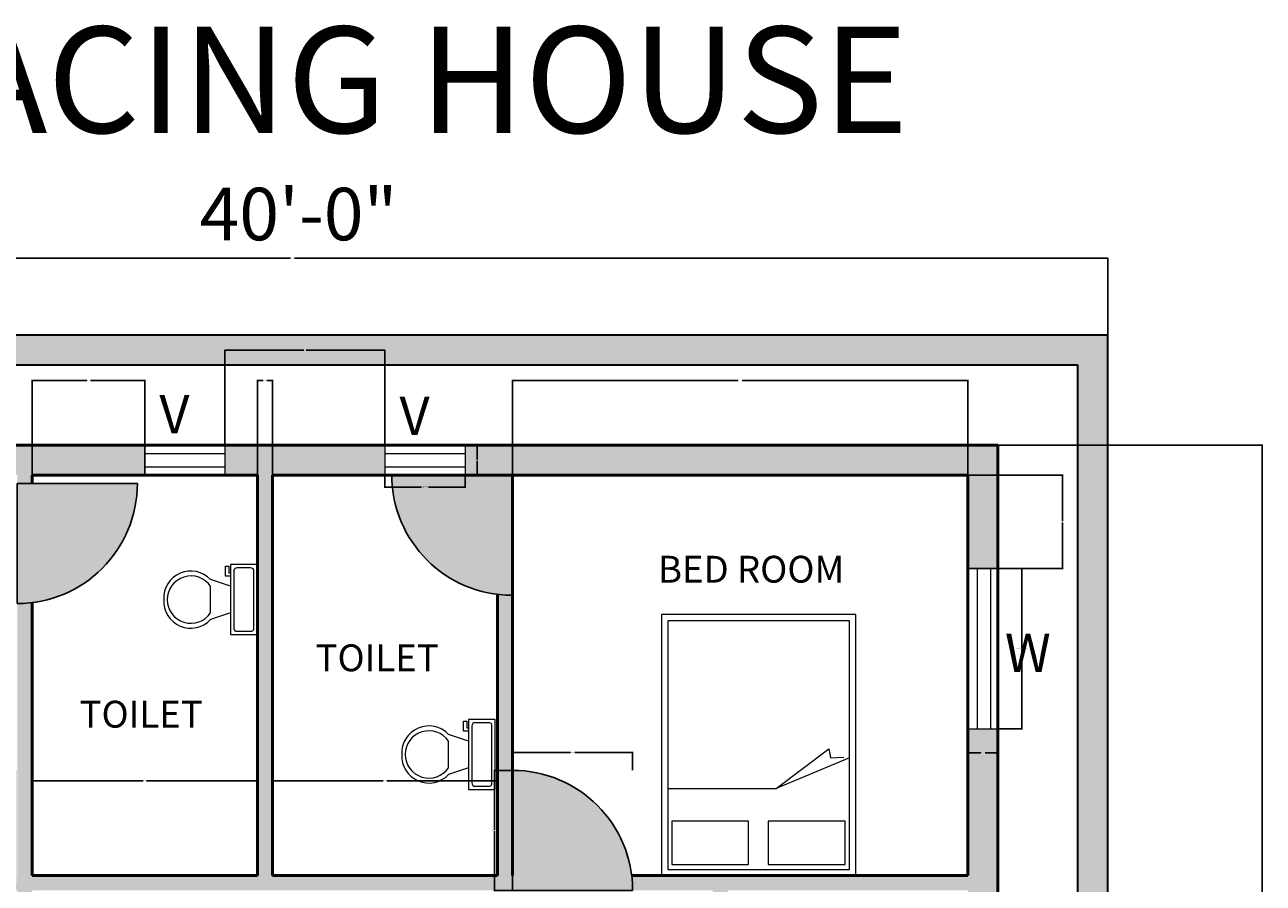
# Model space of a CAD drawing. Units: inches. Extents: x -48 to 546, y -53 to 467.
# Tile 3 of 3: x 174 to 546, y 210 to 467. Entities that reach past the tile are written whole.
import ezdxf

# ---------------------------------------------------------------- set-up
doc = ezdxf.new("R2010")
doc.units = ezdxf.units.IN
doc.header["$MEASUREMENT"] = 0
for name, color, linetype, lineweight in [('A-ANNO-DIMS', 2, 'Continuous', 18), ('A-ANNO-TEXT', 7, 'Continuous', 18), ('A-AREA-IDEN', 7, 'Continuous', 25), ('A-DOOR', 4, 'Continuous', 25), ('A-FLOR-FIXT', 9, 'Continuous', 18), ('A-FURN', 8, 'Continuous', 18), ('A-GLAZ', 4, 'Continuous', 18), ('A-WALL', 7, 'Continuous', 50), ('C-PROP', 7, 'Continuous', 35)]:
    doc.layers.add(name, color=color, linetype=linetype, lineweight=lineweight)
for name, color, linetype, lineweight, true_color in [('A-FLOR-PATT', 253, 'Continuous', 13, 0x9898cc), ('A-WALL-PATT', 251, 'Continuous', 13, 0x636466), ('C-PROP-PATT', 251, 'Continuous', 13, 0x636466)]:
    doc.layers.add(name, color=color, linetype=linetype, lineweight=lineweight, true_color=true_color)
doc.styles.get("Standard").update_dxf_attribs({"font": 'arial.ttf'})
doc.dimstyles.get("Standard").update_dxf_attribs({"dimtxt": 0.18, "dimasz": 0.18, "dimexe": 0.18, "dimexo": 0.0625, "dimgap": 0.09, "dimtad": 0, "dimtih": 1, "dimtoh": 1, "dimdec": 4, "dimzin": 0, "dimdsep": 46, "dimtxsty": 'Standard', "dimcen": 0.09, "dimadec": 0, "dimazin": 0, "dimtfac": 1, "dimtdec": 4, "dimtofl": 0, "dimtmove": 0, "dimatfit": 3, "dimfxl": 1, "dimtolj": 1, "dimtzin": 0, "dimarcsym": 0})

# ---------------------------------------------------------------- blocks, each defined once
blk = doc.blocks.new('*U2')
for p, q in [((9.5, -6), (9.5, -2)), ((-10, -8.5), (-8, -8.5)), ((-10, -9.5), (-10, -8.5)), ((-7, -9.5), (-10, -9.5)), ((-8, -8.5), (-8, -8)), ((-7, -8), (-7, -9.5)), ((-4, -8), (-6, -14)), ((4, -8), (6, -14)), ((4, -14), (-4, -14))]:
    blk.add_line(p, q)
blk.add_lwpolyline([(10.5, -8), (10.5, 0), (-10.5, 0), (-10.5, -8)], close=True)
for points in [[(-9.5, -2), (-9.5, -6)], [(8.5, -1), (-8.5, -1)], [(-8.5, -7), (8.5, -7)]]:
    blk.add_lwpolyline(points)
for centre, radius, start, end in [((-8.625, -1.875), 0.8839, 81.8699, 188.1301), ((8.625, -1.875), 0.8839, 351.8699, 98.1301), ((-8.625, -6.125), 0.8839, 171.869898, 278.1301), ((8.625, -6.125), 0.8839, 261.8699, 8.1301), ((-0.4772, -19.9188), 8.0953, 133.01722, 273.38), ((0.0374, -19.8731), 7.127, 124.50543, 269.7), ((-0.0373, -19.8731), 7.127, 270.3, 55.4946), ((0.4773, -19.9188), 8.0953, 266.62, 46.9828)]:
    blk.add_arc(centre, radius, start, end)
blk = doc.blocks.new('*D3')
at = {"layer": 'A-ANNO-DIMS', "color": 0, "lineweight": -2, "transparency": 16777216}
for p, q in [((10.2, 374.58), (10.2, 397.68)), ((10.38, 397.5), (254.09, 397.5)), ((499.02, 397.5), (255.31, 397.5)), ((499.2, 374.58), (499.2, 397.68))]:
    blk.add_line(p, q, dxfattribs=at)
at = {"layer": 'A-ANNO-DIMS', "color": 0, "transparency": 16777216}
for points in [[(10.38, 397.53), (10.38, 397.47), (10.2, 397.5)], [(499.02, 397.53), (499.02, 397.47), (499.2, 397.5)]]:
    blk.add_solid(points, dxfattribs=at)
at = {"layer": 'Defpoints', "color": 0, "transparency": 16777216}
for p in [(499.2, 397.5), (10.2, 374.51), (499.2, 374.51)]:
    blk.add_point(p, dxfattribs=at)
at = {"layer": 'A-ANNO-DIMS', "color": 0, "transparency": 16777216, "insert": (254.7, 397.5), "char_height": 0.18, "width": 0.9058, "attachment_point": 5}
blk.add_mtext('\\A1;489.0000', dxfattribs=at)
blk = doc.blocks.new('DOOR-SWING-36IN')
for p, q in [((0, 36), (0, 0)), ((0, 0), (36, 0))]:
    blk.add_line(p, q)
blk.add_arc((0, 0), 36, 0, 90)
blk = doc.blocks.new('BED-DOUBLE')
for p, q in [((34.35, 26.2), (50.2, 38.16)), ((50.2, 38.16), (50.65, 35.43)), ((56.35, 35.37), (34.37, 26.2)), ((50.65, 35.43), (54.7, 35.6)), ((1.91, 26.2), (34.35, 26.2))]:
    blk.add_line(p, q)
for points in [[(0, 0), (58.3, 0), (58.3, 78.39), (0, 78.39)], [(1.9, 1.9), (56.4, 1.9), (56.4, 76.49), (1.9, 76.49)], [(3.12, 3.4), (26.1, 3.4), (26.1, 16.4), (3.12, 16.4)], [(32.03, 3.4), (55.02, 3.4), (55.02, 16.4), (32.03, 16.4)]]:
    blk.add_lwpolyline(points, close=True)
blk = doc.blocks.new('VENT-24IN')
for p, q in [((0, 9), (0, 0)), ((24, 9), (24, 0)), ((0, 6.5), (24, 6.5)), ((0, 2.5), (24, 2.5))]:
    blk.add_line(p, q)
blk = doc.blocks.new('WIN-48IN-BEDROOM')
for p, q in [((0, 48), (9, 48)), ((2.8, 48), (2.8, 0)), ((6.8, 48), (6.8, 0)), ((6.8, 48), (6.8, 0)), ((6.8, 48), (6.8, 0)), ((0, 0), (9, 0))]:
    blk.add_line(p, q)
blk = doc.blocks.new('*D14')
at = {"layer": 'A-ANNO-DIMS', "color": 0, "lineweight": -2, "transparency": 16777216}
for p, q in [((320.64, 244.01), (315.12, 244.01)), ((315.3, 243.83), (315.3, 226.2)), ((315.3, 208.19), (315.3, 225.83)), ((320.64, 208.01), (315.12, 208.01))]:
    blk.add_line(p, q, dxfattribs=at)
at = {"layer": 'A-ANNO-DIMS', "color": 0, "transparency": 16777216}
for points in [[(315.27, 243.83), (315.33, 243.83), (315.3, 244.01)], [(315.27, 208.19), (315.33, 208.19), (315.3, 208.01)]]:
    blk.add_solid(points, dxfattribs=at)
at = {"layer": 'Defpoints', "color": 0, "transparency": 16777216}
for p in [(315.3, 244.01), (320.7, 244.01), (320.7, 208.01)]:
    blk.add_point(p, dxfattribs=at)
at = {"layer": 'A-ANNO-DIMS', "color": 0, "transparency": 16777216, "insert": (315.3, 226.01), "char_height": 0.18, "attachment_point": 5}
blk.add_mtext('\\A1;DOOR 3\'-0" TYP.', dxfattribs=at)
blk = doc.blocks.new('*D15')
at = {"layer": 'A-ANNO-DIMS', "color": 0, "lineweight": -2, "transparency": 16777216}
for p, q in [((320.7, 244.08), (320.7, 249.59)), ((320.88, 249.41), (338.06, 249.41)), ((356.52, 249.41), (339.34, 249.41)), ((356.7, 244.08), (356.7, 249.59))]:
    blk.add_line(p, q, dxfattribs=at)
at = {"layer": 'A-ANNO-DIMS', "color": 0, "transparency": 16777216}
for points in [[(320.88, 249.44), (320.88, 249.38), (320.7, 249.41)], [(356.52, 249.44), (356.52, 249.38), (356.7, 249.41)]]:
    blk.add_solid(points, dxfattribs=at)
at = {"layer": 'Defpoints', "color": 0, "transparency": 16777216}
for p in [(356.7, 249.41), (320.7, 244.01), (356.7, 244.01)]:
    blk.add_point(p, dxfattribs=at)
at = {"layer": 'A-ANNO-DIMS', "color": 0, "transparency": 16777216, "insert": (338.7, 249.41), "char_height": 0.18, "attachment_point": 5}
blk.add_mtext('\\A1;3\'-0" TYP.', dxfattribs=at)
blk = doc.blocks.new('*D16')
at = {"layer": 'A-ANNO-DIMS', "color": 0, "lineweight": -2, "transparency": 16777216}
for p, q in [((282.45, 332.45), (282.45, 328.73)), ((306.45, 332.45), (306.45, 328.73)), ((282.63, 328.91), (293.44, 328.91)), ((306.27, 328.91), (295.46, 328.91))]:
    blk.add_line(p, q, dxfattribs=at)
at = {"layer": 'A-ANNO-DIMS', "color": 0, "transparency": 16777216}
for points in [[(282.63, 328.94), (282.63, 328.88), (282.45, 328.91)], [(306.27, 328.94), (306.27, 328.88), (306.45, 328.91)]]:
    blk.add_solid(points, dxfattribs=at)
at = {"layer": 'Defpoints', "color": 0, "transparency": 16777216}
for p in [(282.45, 332.51), (306.45, 332.51), (306.45, 328.91)]:
    blk.add_point(p, dxfattribs=at)
at = {"layer": 'A-ANNO-DIMS', "color": 0, "transparency": 16777216, "insert": (294.45, 328.91), "char_height": 0.18, "attachment_point": 5}
blk.add_mtext('\\A1;VENT 2\'-0" TYP.', dxfattribs=at)
blk = doc.blocks.new('*D17')
at = {"layer": 'A-ANNO-DIMS', "color": 0, "lineweight": -2, "transparency": 16777216}
for p, q in [((306.51, 341.51), (310.23, 341.51)), ((310.05, 341.33), (310.05, 337.2)), ((310.05, 332.69), (310.05, 336.83)), ((306.51, 332.51), (310.23, 332.51))]:
    blk.add_line(p, q, dxfattribs=at)
at = {"layer": 'A-ANNO-DIMS', "color": 0, "transparency": 16777216}
for points in [[(310.02, 341.33), (310.08, 341.33), (310.05, 341.51)], [(310.02, 332.69), (310.08, 332.69), (310.05, 332.51)]]:
    blk.add_solid(points, dxfattribs=at)
at = {"layer": 'Defpoints', "color": 0, "transparency": 16777216}
for p in [(306.45, 341.51), (310.05, 341.51), (306.45, 332.51)]:
    blk.add_point(p, dxfattribs=at)
at = {"layer": 'A-ANNO-DIMS', "color": 0, "transparency": 16777216, "insert": (310.05, 337.01), "char_height": 0.18, "attachment_point": 5}
blk.add_mtext('\\A1;0\'-9" TYP.', dxfattribs=at)
blk = doc.blocks.new('*D20')
at = {"layer": 'A-ANNO-DIMS', "color": 0, "lineweight": -2, "transparency": 16777216}
for p, q in [((466.26, 304.5), (473.58, 304.5)), ((473.4, 304.32), (473.4, 280.68)), ((473.4, 256.68), (473.4, 280.32)), ((466.26, 256.5), (473.58, 256.5))]:
    blk.add_line(p, q, dxfattribs=at)
at = {"layer": 'A-ANNO-DIMS', "color": 0, "transparency": 16777216}
for points in [[(473.37, 304.32), (473.43, 304.32), (473.4, 304.5)], [(473.37, 256.68), (473.43, 256.68), (473.4, 256.5)]]:
    blk.add_solid(points, dxfattribs=at)
at = {"layer": 'Defpoints', "color": 0, "transparency": 16777216}
for p in [(466.2, 304.5), (473.4, 304.5), (466.2, 256.5)]:
    blk.add_point(p, dxfattribs=at)
at = {"layer": 'A-ANNO-DIMS', "color": 0, "transparency": 16777216, "insert": (473.4, 280.5), "char_height": 0.18, "attachment_point": 5}
blk.add_mtext('\\A1;BEDROOM WINDOW 4\'-0" TYP.', dxfattribs=at)
blk = doc.blocks.new('*D21')
at = {"layer": 'A-ANNO-DIMS', "color": 0, "lineweight": -2, "transparency": 16777216}
for p, q in [((457.2, 256.44), (457.2, 249.12)), ((466.2, 256.44), (466.2, 249.12)), ((457.38, 249.3), (461.06, 249.3)), ((466.02, 249.3), (462.34, 249.3))]:
    blk.add_line(p, q, dxfattribs=at)
at = {"layer": 'A-ANNO-DIMS', "color": 0, "transparency": 16777216}
for points in [[(457.38, 249.33), (457.38, 249.27), (457.2, 249.3)], [(466.02, 249.33), (466.02, 249.27), (466.2, 249.3)]]:
    blk.add_solid(points, dxfattribs=at)
at = {"layer": 'Defpoints', "color": 0, "transparency": 16777216}
for p in [(457.2, 256.5), (466.2, 256.5), (466.2, 249.3)]:
    blk.add_point(p, dxfattribs=at)
at = {"layer": 'A-ANNO-DIMS', "color": 0, "transparency": 16777216, "insert": (461.7, 249.3), "char_height": 0.18, "attachment_point": 5}
blk.add_mtext('\\A1;0\'-9" TYP.', dxfattribs=at)
blk = doc.blocks.new('*D27')
at = {"layer": 'A-ANNO-DIMS', "color": 0, "lineweight": -2, "transparency": 16777216}
for p, q in [((466.26, 341.51), (545.59, 341.51)), ((545.41, 341.33), (545.41, 190.2)), ((545.41, 38.69), (545.41, 189.83)), ((466.26, 38.51), (545.59, 38.51))]:
    blk.add_line(p, q, dxfattribs=at)
at = {"layer": 'A-ANNO-DIMS', "color": 0, "transparency": 16777216}
for points in [[(545.38, 341.33), (545.44, 341.33), (545.41, 341.51)], [(545.38, 38.69), (545.44, 38.69), (545.41, 38.51)]]:
    blk.add_solid(points, dxfattribs=at)
at = {"layer": 'Defpoints', "color": 0, "transparency": 16777216}
for p in [(466.2, 341.51), (545.41, 341.51), (466.2, 38.51)]:
    blk.add_point(p, dxfattribs=at)
at = {"layer": 'A-ANNO-DIMS', "color": 0, "transparency": 16777216, "insert": (545.41, 190.01), "char_height": 0.18, "attachment_point": 5}
blk.add_mtext('\\A1;25\'-3"', dxfattribs=at)
blk = doc.blocks.new('*D31')
at = {"layer": 'A-ANNO-DIMS', "color": 0, "lineweight": -2, "transparency": 16777216}
for p, q in [((176.7, 212.58), (176.7, 241.09)), ((176.88, 240.91), (209.91, 240.91)), ((244.02, 240.91), (210.99, 240.91)), ((244.2, 212.58), (244.2, 241.09))]:
    blk.add_line(p, q, dxfattribs=at)
at = {"layer": 'A-ANNO-DIMS', "color": 0, "transparency": 16777216}
for points in [[(176.88, 240.94), (176.88, 240.88), (176.7, 240.91)], [(244.02, 240.94), (244.02, 240.88), (244.2, 240.91)]]:
    blk.add_solid(points, dxfattribs=at)
at = {"layer": 'Defpoints', "color": 0, "transparency": 16777216}
for p in [(244.2, 240.91), (176.7, 212.51), (244.2, 212.51)]:
    blk.add_point(p, dxfattribs=at)
at = {"layer": 'A-ANNO-DIMS', "color": 0, "transparency": 16777216, "insert": (210.45, 240.91), "char_height": 0.18, "attachment_point": 5}
blk.add_mtext('\\A1;5\'-7 1/2"', dxfattribs=at)
blk = doc.blocks.new('*D32')
at = {"layer": 'A-ANNO-DIMS', "color": 0, "lineweight": -2, "transparency": 16777216}
for p, q in [((248.7, 212.58), (248.7, 241.09)), ((248.88, 240.91), (281.91, 240.91)), ((316.02, 240.91), (282.99, 240.91)), ((316.2, 212.58), (316.2, 241.09))]:
    blk.add_line(p, q, dxfattribs=at)
at = {"layer": 'A-ANNO-DIMS', "color": 0, "transparency": 16777216}
for points in [[(248.88, 240.94), (248.88, 240.88), (248.7, 240.91)], [(316.02, 240.94), (316.02, 240.88), (316.2, 240.91)]]:
    blk.add_solid(points, dxfattribs=at)
at = {"layer": 'Defpoints', "color": 0, "transparency": 16777216}
for p in [(316.2, 240.91), (248.7, 212.51), (316.2, 212.51)]:
    blk.add_point(p, dxfattribs=at)
at = {"layer": 'A-ANNO-DIMS', "color": 0, "transparency": 16777216, "insert": (282.45, 240.91), "char_height": 0.18, "attachment_point": 5}
blk.add_mtext('\\A1;5\'-7 1/2"', dxfattribs=at)
blk = doc.blocks.new('*D33')
at = {"layer": 'A-ANNO-DIMS', "color": 0, "lineweight": -2, "transparency": 16777216}
for p, q in [((320.7, 332.58), (320.7, 361.09)), ((320.88, 360.91), (388.35, 360.91)), ((457.02, 360.91), (389.55, 360.91)), ((457.2, 332.58), (457.2, 361.09))]:
    blk.add_line(p, q, dxfattribs=at)
at = {"layer": 'A-ANNO-DIMS', "color": 0, "transparency": 16777216}
for points in [[(320.88, 360.94), (320.88, 360.88), (320.7, 360.91)], [(457.02, 360.94), (457.02, 360.88), (457.2, 360.91)]]:
    blk.add_solid(points, dxfattribs=at)
at = {"layer": 'Defpoints', "color": 0, "transparency": 16777216}
for p in [(457.2, 360.91), (320.7, 332.51), (457.2, 332.51)]:
    blk.add_point(p, dxfattribs=at)
at = {"layer": 'A-ANNO-DIMS', "color": 0, "transparency": 16777216, "insert": (388.95, 360.91), "char_height": 0.18, "attachment_point": 5}
blk.add_mtext('\\A1;11\'-4 1/2"', dxfattribs=at)
blk = doc.blocks.new('*D43')
at = {"layer": 'A-ANNO-DIMS', "color": 0, "lineweight": -2, "transparency": 16777216}
for p, q in [((457.26, 332.51), (485.78, 332.51)), ((485.6, 332.33), (485.6, 318.69)), ((485.6, 304.68), (485.6, 318.33)), ((457.26, 304.5), (485.78, 304.5))]:
    blk.add_line(p, q, dxfattribs=at)
at = {"layer": 'A-ANNO-DIMS', "color": 0, "transparency": 16777216}
for points in [[(485.57, 332.33), (485.63, 332.33), (485.6, 332.51)], [(485.57, 304.68), (485.63, 304.68), (485.6, 304.5)]]:
    blk.add_solid(points, dxfattribs=at)
at = {"layer": 'Defpoints', "color": 0, "transparency": 16777216}
for p in [(457.2, 332.51), (457.2, 304.5), (485.6, 304.5)]:
    blk.add_point(p, dxfattribs=at)
at = {"layer": 'A-ANNO-DIMS', "color": 0, "transparency": 16777216, "insert": (485.6, 318.51), "char_height": 0.18, "attachment_point": 5}
blk.add_mtext('\\A1;2\'-4"', dxfattribs=at)
blk = doc.blocks.new('*D46')
at = {"layer": 'A-ANNO-DIMS', "color": 0, "lineweight": -2, "transparency": 16777216}
for p, q in [((176.7, 332.58), (176.7, 361.09)), ((176.88, 360.91), (193.03, 360.91)), ((210.27, 360.91), (194.12, 360.91)), ((210.45, 332.58), (210.45, 361.09))]:
    blk.add_line(p, q, dxfattribs=at)
at = {"layer": 'A-ANNO-DIMS', "color": 0, "transparency": 16777216}
for points in [[(176.88, 360.94), (176.88, 360.88), (176.7, 360.91)], [(210.27, 360.94), (210.27, 360.88), (210.45, 360.91)]]:
    blk.add_solid(points, dxfattribs=at)
at = {"layer": 'Defpoints', "color": 0, "transparency": 16777216}
for p in [(210.45, 360.91), (176.7, 332.51), (210.45, 332.51)]:
    blk.add_point(p, dxfattribs=at)
at = {"layer": 'A-ANNO-DIMS', "color": 0, "transparency": 16777216, "insert": (193.57, 360.91), "char_height": 0.18, "attachment_point": 5}
blk.add_mtext('\\A1;2\'-9 1/2"', dxfattribs=at)
blk = doc.blocks.new('*D47')
at = {"layer": 'A-ANNO-DIMS', "color": 0, "lineweight": -2, "transparency": 16777216}
for p, q in [((234.45, 341.58), (234.45, 370.09)), ((234.63, 369.91), (258.12, 369.91)), ((282.27, 369.91), (258.78, 369.91)), ((282.45, 341.58), (282.45, 370.09))]:
    blk.add_line(p, q, dxfattribs=at)
at = {"layer": 'A-ANNO-DIMS', "color": 0, "transparency": 16777216}
for points in [[(234.63, 369.94), (234.63, 369.88), (234.45, 369.91)], [(282.27, 369.94), (282.27, 369.88), (282.45, 369.91)]]:
    blk.add_solid(points, dxfattribs=at)
at = {"layer": 'Defpoints', "color": 0, "transparency": 16777216}
for p in [(282.45, 369.91), (234.45, 341.51), (282.45, 341.51)]:
    blk.add_point(p, dxfattribs=at)
at = {"layer": 'A-ANNO-DIMS', "color": 0, "transparency": 16777216, "insert": (258.45, 369.91), "char_height": 0.18, "attachment_point": 5}
blk.add_mtext('\\A1;4\'-0"', dxfattribs=at)
blk = doc.blocks.new('*D48')
at = {"layer": 'A-ANNO-DIMS', "color": 0, "lineweight": -2, "transparency": 16777216}
for p, q in [((244.2, 332.58), (244.2, 361.09)), ((244.38, 360.91), (245.91, 360.91)), ((248.52, 360.91), (246.99, 360.91)), ((248.7, 332.58), (248.7, 361.09))]:
    blk.add_line(p, q, dxfattribs=at)
at = {"layer": 'A-ANNO-DIMS', "color": 0, "transparency": 16777216}
for points in [[(244.38, 360.94), (244.38, 360.88), (244.2, 360.91)], [(248.52, 360.94), (248.52, 360.88), (248.7, 360.91)]]:
    blk.add_solid(points, dxfattribs=at)
at = {"layer": 'Defpoints', "color": 0, "transparency": 16777216}
for p in [(248.7, 360.91), (244.2, 332.51), (248.7, 332.51)]:
    blk.add_point(p, dxfattribs=at)
at = {"layer": 'A-ANNO-DIMS', "color": 0, "transparency": 16777216, "insert": (246.45, 360.91), "char_height": 0.18, "attachment_point": 5}
blk.add_mtext('\\A1;0\'-4 1/2"', dxfattribs=at)

msp = doc.modelspace()

# ---------------------------------------------------------------- hatches: boundary and pattern name
at = {"layer": 'A-FLOR-PATT'}
h = msp.add_hatch(color=256, dxfattribs=at)
h.dxf.hatch_style = 1
h.paths.add_polyline_path([(208.19994, 330.01344), (172.19994, 330.01344), (172.19994, 294.01344, 0.414213549)])
h.paths.add_polyline_path([(320.5, 332.5), (284.5, 332.5, 0.414213562), (320.5, 296.5)])
h.paths.add_polyline_path([(417, 204.5), (381, 204.5), (381, 168.5, 0.414213562)])
h.paths.add_polyline_path([(177, 74.5), (177, 38.51344), (213, 38.51344, 0.414104244)])
h.paths.add_polyline_path([(172, 244, 0.414104258), (136, 208.01344), (172, 208.01344)])
h.paths.add_polyline_path([(320.69994, 244.01344), (320.69994, 212.51344), (320.69994, 208.01344), (356.69994, 208.01344, 0.414213532)])
h.paths.add_polyline_path([(172.19994, 78.5), (52.19994, 78.5), (52.19994, 47.51344), (172.19994, 47.51344)])
h.paths.add_polyline_path([(126, 74), (166, 74), (166, 54.5), (126, 54.5)], flags=16)
h.paths.add_polyline_path([(101, 53), (56.5, 53), (56.5, 74.5), (101, 74.5)], flags=16)
h.paths.add_polyline_path([(141, 69), (162.5, 69), (162.5, 58.5), (141, 58.5)], flags=0)
h.paths.add_polyline_path([(97.5, 55), (83, 55), (83, 67.5), (97.5, 67.5)], flags=0)
h.paths.add_polyline_path([(84, 61.5, -1), (96, 61.5, -1)], flags=0)
h.paths.add_polyline_path([(88.5, 71.5, -1), (92.5, 71.5, -1)], flags=0)
h.paths.add_polyline_path([(90, 71.5, -1), (91, 71.5, -1)], flags=0)
h.paths.add_polyline_path([(162, 64.5, -1), (158, 64.5, -1)], flags=0)
h.paths.add_polyline_path([(75, 55), (60.5, 55), (60.5, 67.5), (75, 67.5)], flags=0)
h.paths.add_polyline_path([(61.5, 61.5, -1), (73.5, 61.5, -1)], flags=0)
h.paths.add_polyline_path([(66, 71.5, -1), (70, 71.5, -1)], flags=0)
h.paths.add_polyline_path([(67.5, 71.5, -1), (68.5, 71.5, -1)], flags=0)
h.paths.add_polyline_path([(176.42827, 40.63764), (207.16292, 40.63764), (207.16292, 57.88764), (176.42827, 57.88764)], flags=9)
at = {"layer": 'A-WALL-PATT'}
h = msp.add_hatch(color=256, dxfattribs=at)
h.dxf.hatch_style = 1
h.paths.add_polyline_path([(282.44994, 341.51344), (234.44994, 341.51344), (234.44994, 332.51344), (244.19994, 332.51344), (244.19994, 212.51344), (176.69994, 212.51344), (176.69994, 294.29579, -0.031342215), (172.19994, 294.01344), (172.19994, 212.51344), (172.00059, 208.01344), (172.19994, 208.01344), (172.19994, 47.51344), (120, 47.51344), (120, 38.51344), (177, 38.51344), (177, 47.51344), (176.69994, 47.51344), (176.69994, 208.01344), (320.69994, 208.01344), (320.69994, 244.01344), (320.69994, 296.50056, -0.031331714), (316.19994, 296.75774), (316.19994, 212.51344), (248.69994, 212.51344), (248.69994, 332.51344), (282.44994, 332.51344)])
h.paths.add_polyline_path([(466.19994, 341.51344), (306.44994, 341.51344), (306.44994, 332.51344), (316.19994, 332.51344), (457.19994, 332.51344), (457.19994, 304.5), (466.19994, 304.5)])
h.paths.add_polyline_path([(466.19994, 256.5), (457.19994, 256.5), (457.19994, 212.51344), (423.64319, 212.51344), (423.64319, 212.34928), (365.34701, 212.34928), (356.41758, 212.51344, -0.031342215), (356.69994, 208.01344), (380.69994, 208.01344), (380.69994, 204.5), (385.19994, 204.5), (385.19994, 208.01344), (457.19994, 208.01344), (457.19994, 191.5), (466.19994, 191.5)])
h.paths.add_polyline_path([(210.44994, 341.51344), (43.19994, 341.51344), (43.19994, 303.5), (52.19994, 303.5), (52.19994, 332.51344), (172.19994, 332.51344), (172.19994, 330.01344), (176.69994, 330.01344), (176.69994, 332.51344), (210.44994, 332.51344)])
h.paths.add_polyline_path([(52.19994, 208.01344), (136, 208.01344, -0.031342955), (136.28405, 212.51344), (52.19994, 212.51344), (52.19994, 255.5), (43.19994, 255.5), (43.19994, 38.51344), (72, 38.51344), (72, 47.51344), (52.19994, 47.51344)])
h.paths.add_polyline_path([(466.19994, 62.5), (457.19994, 62.5), (457.19994, 47.51344), (380.69994, 47.51344), (263, 47.51344), (263, 38.51344), (466.19994, 38.51344)])
h.paths.add_polyline_path([(215, 47.51344), (211.85338, 47.51344, -0.063257301), (213, 38.51344), (215, 38.51344)])
h.paths.add_polyline_path([(466.19994, 167.5), (457.19994, 167.5), (457.19994, 136.01344), (385.19994, 136.01344), (385.19994, 168.74583, -0.031326837), (380.69994, 168.50125), (380.69994, 131.51344), (457.19994, 131.51344), (457.19994, 110.5), (466.19994, 110.5)])
h = msp.add_hatch(color=256, dxfattribs=at)
h.dxf.hatch_style = 1
h.paths.add_polyline_path([(210.44994, 341.51344), (43.19994, 341.51344), (43.19994, 303.5), (52.19994, 303.5), (52.19994, 332.51344), (172.19994, 332.51344), (172.19994, 330.01344), (176.69994, 330.01344), (176.69994, 332.51344), (210.44994, 332.51344)])
h.paths.add_polyline_path([(466.19994, 341.51344), (306.44994, 341.51344), (306.44994, 332.51344), (316.19994, 332.51344), (457.19994, 332.51344), (457.19994, 304.5), (466.19994, 304.5)])
h.paths.add_polyline_path([(282.44994, 341.51344), (234.44994, 341.51344), (234.44994, 332.51344), (244.19994, 332.51344), (244.19994, 212.51344), (176.69994, 212.51344), (176.69994, 294.29579, -0.031342215), (172.19994, 294.01344), (172.19994, 212.51344), (172.00059, 208.01344), (172.19994, 208.01344), (172.19994, 47.51344), (120, 47.51344), (120, 38.51344), (177, 38.51344), (177, 47.51344), (176.69994, 47.51344), (176.69994, 208.01344), (320.69994, 208.01344), (320.69994, 244.01344), (320.69994, 296.50056, -0.031331714), (316.19994, 296.75774), (316.19994, 212.51344), (248.69994, 212.51344), (248.69994, 332.51344), (282.44994, 332.51344)])
h.paths.add_polyline_path([(52.19994, 255.5), (43.19994, 255.5), (43.19994, 38.51344), (72, 38.51344), (72, 47.51344), (52.19994, 47.51344), (52.19994, 208.01344), (136, 208.01344, -0.031342955), (136.28405, 212.51344), (52.19994, 212.51344)])
h.paths.add_polyline_path([(466.19994, 256.5), (457.19994, 256.5), (457.19994, 212.51344), (423.64319, 212.51344), (423.64319, 212.34928), (365.34701, 212.34928), (356.41758, 212.51344, -0.031342215), (356.69994, 208.01344), (380.69994, 208.01344), (380.69994, 204.5), (385.19994, 204.5), (385.19994, 208.01344), (457.19994, 208.01344), (457.19994, 191.5), (466.19994, 191.5)])
h.paths.add_polyline_path([(466.19994, 167.5), (457.19994, 167.5), (457.19994, 136.01344), (385.19994, 136.01344), (385.19994, 168.74583, -0.031326837), (380.69994, 168.50125), (380.69994, 131.51344), (457.19994, 131.51344), (457.19994, 110.5), (466.19994, 110.5)])
h.paths.add_polyline_path([(466.19994, 62.5), (457.19994, 62.5), (457.19994, 47.51344), (380.69994, 47.51344), (263, 47.51344), (263, 38.51344), (466.19994, 38.51344)])
h.paths.add_polyline_path([(215, 47.51344), (211.85338, 47.51344, -0.063257301), (213, 38.51344), (215, 38.51344)])
at = {"layer": 'C-PROP-PATT'}
h = msp.add_hatch(color=256, dxfattribs=at)
h.dxf.hatch_style = 1
h.paths.add_polyline_path([(499.19994, 374.51344), (10.19994, 374.51344), (10.19994, 5.51344), (103, 5.51344), (103, 14.51344), (19.19994, 14.51344), (19.19994, 365.51344), (490.19994, 365.51344), (490.19994, 14.51344), (192.5, 14.51344), (192.5, 5.51344), (499.19994, 5.51344)])

# ---------------------------------------------------------------- linework, layer by layer
at = {"layer": 'A-WALL'}
for p, q in [((43.19994, 341.51344), (466.19994, 341.51344)), ((466.19994, 38.51344), (466.19994, 341.51344)), ((176.69994, 332.51344), (244.19994, 332.51344)), ((176.69994, 330.01344), (176.69994, 332.51344)), ((244.19994, 212.51344), (244.19994, 332.51344)), ((248.69994, 212.51344), (248.69994, 332.51344)), ((248.69994, 332.51344), (316.19994, 332.51344)), ((316.19994, 332.51344), (457.19994, 332.51344)), ((316.19994, 332.5), (316.19994, 332.51344)), ((320.69994, 212.51344), (320.69994, 332.51344)), ((457.19994, 212.51344), (457.19994, 332.51344)), ((176.69994, 212.51344), (176.69994, 294.29579)), ((316.19994, 212.51344), (316.19994, 296.75774)), ((176.69994, 212.51344), (244.19994, 212.51344)), ((248.69994, 212.51344), (316.19994, 212.51344)), ((356.41758, 212.51344), (457.19994, 212.51344))]:
    msp.add_line(p, q, dxfattribs=at)
at = {"layer": 'C-PROP'}
for p, q in [((10.19994, 374.51344), (499.19994, 374.51344)), ((499.19994, 5.51344), (499.19994, 374.51344)), ((19.19994, 365.51344), (490.19994, 365.51344)), ((490.19994, 14.51344), (490.19994, 365.51344))]:
    msp.add_line(p, q, dxfattribs=at)

# ---------------------------------------------------------------- block references
at = {"layer": 'A-DOOR'}
for p, rotation in [((320.49994, 332.50044), 180), ((172.19951, 330.01338), 270.0000000000002)]:
    msp.add_blockref('DOOR-SWING-36IN', p, dxfattribs=dict(at, rotation=rotation))
msp.add_blockref('DOOR-SWING-36IN', (320.7, 208.013), dxfattribs=at)
at = {"layer": 'A-FLOR-FIXT', "rotation": 270}
for p in [(244.14054, 295.19249), (315.49814, 248.77019)]:
    msp.add_blockref('*U2', p, dxfattribs=at)
at = {"layer": 'A-FURN'}
msp.add_blockref('BED-DOUBLE', (365.34702, 212.34958), dxfattribs=at)
at = {"layer": 'A-GLAZ'}
for name, p in [('VENT-24IN', (210.45, 332.513)), ('VENT-24IN', (282.45, 332.513)), ('WIN-48IN-BEDROOM', (457.2, 256.5))]:
    msp.add_blockref(name, p, dxfattribs=at)

# ---------------------------------------------------------------- texts
at = {"layer": 'A-ANNO-DIMS'}
msp.add_text('40\'-0"', height=15.736247, dxfattribs=at).set_placement((226.8508, 402.89558))
at = {"layer": 'A-ANNO-TEXT'}
for s, height, p in [('EAST FACING HOUSE', 31.8325196, (17.25357, 435.09398)), ('V', 11.5, (214.80327, 345.01264)), ('V', 11.5, (286.80327, 344.51264)), ('W', 11.5, (468.30327, 273.51264))]:
    msp.add_text(s, height=height, dxfattribs=at).set_placement(p)
at = {"layer": 'A-AREA-IDEN'}
for s, p in [('BED ROOM', (364.28997, 300.27992)), ('TOILET', (261.6446, 273.71862)), ('TOILET', (190.89139, 256.82544))]:
    msp.add_text(s, height=8.042128, dxfattribs=at).set_placement(p)

# ---------------------------------------------------------------- dimensions: what is measured, and where the dimension line sits
at = {"layer": 'A-ANNO-DIMS'}
for base, p1, p2, override, picture, middle in [((499.19994, 397.5), (10.19994, 374.51344), (499.19994, 374.51344), {"dimclrd": 0, "dimclre": 0, "dimclrt": 0}, '*D3', (254.69994, 397.5)), ((282.44994, 369.91344), (234.44994, 341.51344), (282.44994, 341.51344), {"dimdec": 1, "dimlfac": 1, "dimrnd": 0, "dimzin": 1, "dimdsep": 46, "dimlunit": 4, "dimfrac": 2}, '*D47', (258.44994, 369.91344)), ((248.69994, 360.91344), (244.19994, 332.51344), (248.69994, 332.51344), {"dimdec": 1, "dimlfac": 1, "dimrnd": 0, "dimzin": 1, "dimdsep": 46, "dimlunit": 4, "dimfrac": 2}, '*D48', (246.44994, 360.91344)), ((244.19994, 240.91344), (176.69994, 212.51344), (244.19994, 212.51344), {"dimdec": 1, "dimlfac": 1, "dimrnd": 0, "dimzin": 1, "dimdsep": 46, "dimlunit": 4, "dimfrac": 2}, '*D31', (210.44994, 240.91344)), ((316.19994, 240.91344), (248.69994, 212.51344), (316.19994, 212.51344), {"dimdec": 1, "dimlfac": 1, "dimrnd": 0, "dimzin": 1, "dimdsep": 46, "dimlunit": 4, "dimfrac": 2}, '*D32', (282.44994, 240.91344))]:
    dim = msp.add_linear_dim(base=base, p1=p1, p2=p2, dimstyle='Standard', override=override, dxfattribs=at)
    dim.commit()
    dim.dimension.update_dxf_attribs({"geometry": picture, "text_midpoint": middle})
for base, p1, p2, angle, picture, middle in [((210.449937, 360.913437), (176.699943, 332.513436), (210.449937, 332.513438), 0.0000032, '*D46', (193.57494, 360.913437)), ((457.19994, 360.91344), (320.69994, 332.51344), (457.19994, 332.51344), 0, '*D33', (388.94994, 360.91344)), ((545.41404, 341.51344), (466.19994, 38.51344), (466.19994, 341.51344), 90, '*D27', (545.41404, 190.01344)), ((485.59994, 304.5), (457.19994, 332.51344), (457.19994, 304.5), 270, '*D43', (485.59994, 318.50672))]:
    dim = msp.add_linear_dim(base=base, p1=p1, p2=p2, angle=angle, dimstyle='Standard', override={"dimdec": 1, "dimlfac": 1, "dimrnd": 0, "dimzin": 1, "dimdsep": 46, "dimlunit": 4, "dimfrac": 2}, dxfattribs=at)
    dim.commit()
    dim.dimension.update_dxf_attribs({"geometry": picture, "text_midpoint": middle})
for base, p1, p2, text, picture, middle in [((310.04994, 341.51344), (306.44994, 332.51344), (306.44994, 341.51344), '<> TYP.', '*D17', (310.04994, 337.01344)), ((473.39994, 304.5), (466.19994, 256.5), (466.19994, 304.5), 'BEDROOM WINDOW <> TYP.', '*D20', (473.39994, 280.5)), ((315.29994, 244.01344), (320.69994, 208.01344), (320.69994, 244.01344), 'DOOR <> TYP.', '*D14', (315.29994, 226.01344))]:
    dim = msp.add_linear_dim(base=base, p1=p1, p2=p2, angle=90, text=text, dimstyle='Standard', override={"dimdec": 1, "dimlfac": 1, "dimrnd": 0, "dimzin": 1, "dimdsep": 46, "dimlunit": 4, "dimfrac": 2}, dxfattribs=at)
    dim.commit()
    dim.dimension.update_dxf_attribs({"geometry": picture, "text_midpoint": middle})
for base, p1, p2, text, picture, middle in [((306.44994, 328.91344), (282.44994, 332.51344), (306.44994, 332.51344), 'VENT <> TYP.', '*D16', (294.44994, 328.91344)), ((466.19994, 249.3), (457.19994, 256.5), (466.19994, 256.5), '<> TYP.', '*D21', (461.69994, 249.3)), ((356.69994, 249.41344), (320.69994, 244.01344), (356.69994, 244.01344), '<> TYP.', '*D15', (338.69994, 249.41344))]:
    dim = msp.add_linear_dim(base=base, p1=p1, p2=p2, text=text, dimstyle='Standard', override={"dimdec": 1, "dimlfac": 1, "dimrnd": 0, "dimzin": 1, "dimdsep": 46, "dimlunit": 4, "dimfrac": 2}, dxfattribs=at)
    dim.commit()
    dim.dimension.update_dxf_attribs({"geometry": picture, "text_midpoint": middle})

doc.saveas('drawing.dxf')
